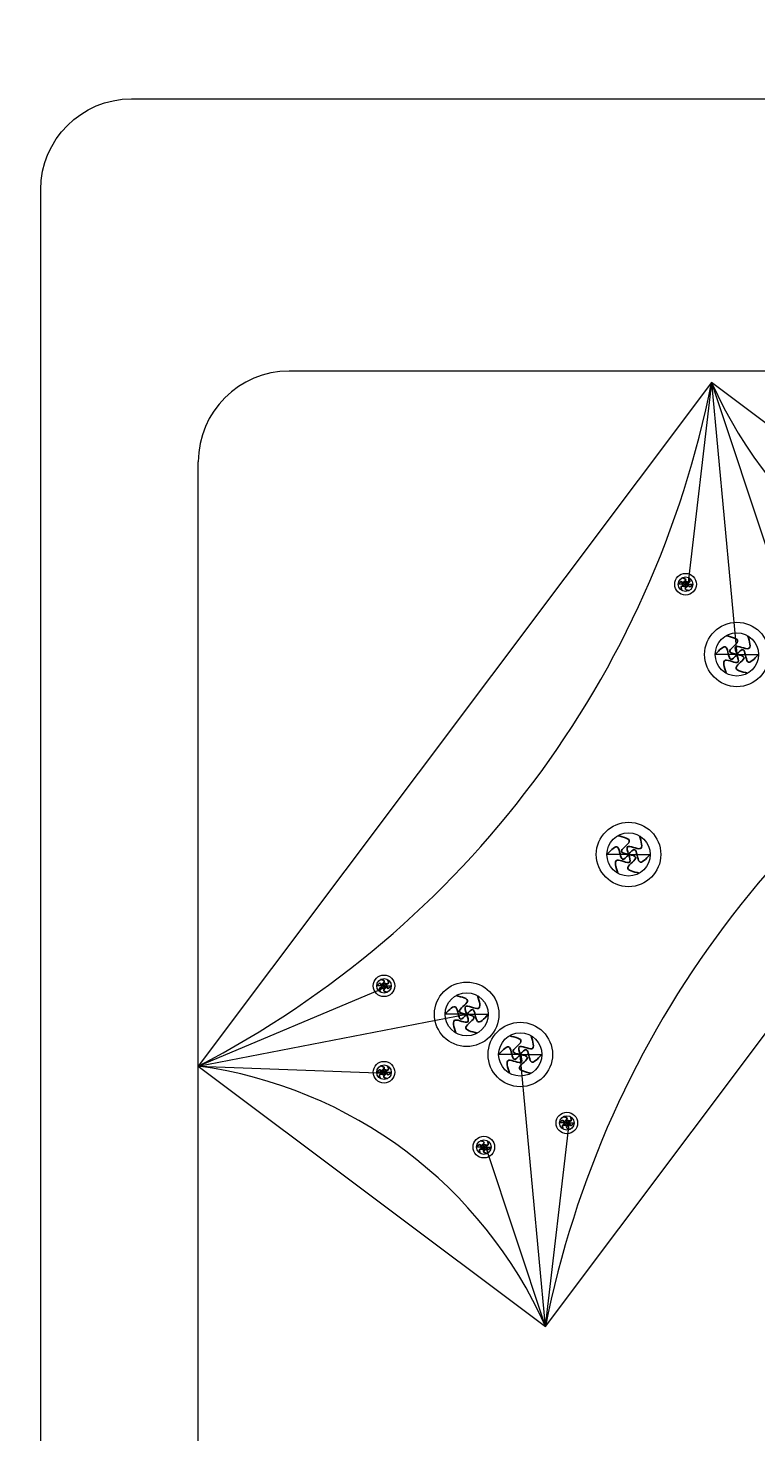
# Model space of a CAD drawing. Units: inches. Extents: x -61 to 1599, y -1316 to 257.
# Tile 103 of 204: x 126 to 142, y -99 to -68. Entities that reach past the tile are written whole.
import ezdxf

# ---------------------------------------------------------------- set-up
doc = ezdxf.new("R2010")
doc.units = ezdxf.units.IN
doc.header["$MEASUREMENT"] = 0
doc.layers.add('A-ANNO-DIMS', color=2, linetype='Continuous', lineweight=18)
doc.layers.add('FURNITURE', color=83, linetype='Continuous', lineweight=18)
doc.layers.add('FUR', color=83, linetype='Continuous')
doc.styles.get("Standard").update_dxf_attribs({"font": 'arial.ttf'})
doc.dimstyles.get("Standard").update_dxf_attribs({"dimtxt": 0.18, "dimasz": 0.18, "dimexe": 0.18, "dimexo": 0.0625, "dimgap": 0.09, "dimtad": 0, "dimtih": 1, "dimtoh": 1, "dimdec": 0, "dimzin": 0, "dimdsep": 46, "dimlunit": 3, "dimtxsty": 'Standard', "dimcen": 0.09, "dimadec": 0, "dimazin": 0, "dimtfac": 1, "dimtdec": 0, "dimtofl": 0, "dimtmove": 0, "dimatfit": 3, "dimfxl": 1, "dimtolj": 1, "dimtzin": 0, "dimarcsym": 0})

# ---------------------------------------------------------------- blocks, each defined once
blk = doc.blocks.new('*U186')
at = {"layer": 'FUR'}
blk.add_open_spline([(0.005, 0.08), (-0.03, 0.048), (-0.098, -0.015), (0.075, -0.018), (0.024, -0.063), (0.005, -0.08)], degree=3, knots=[0, 0, 0, 0, 0.0954578, 0.1898773, 0.2470677, 0.2470677, 0.2470677, 0.2470677], dxfattribs=at)
blk = doc.blocks.new('*U187')
at = {"layer": 'FUR', "transparency": 16777216}
for p, rotation in [((222.173, -79.977), 60), ((222.178, -80.056), 120), ((222.25, -80.092), 180), ((222.312, -79.968), 300), ((222.317, -80.048), 240)]:
    blk.add_blockref('*U186', p, dxfattribs=dict(at, rotation=rotation))
blk.add_blockref('*U186', (222.24, -79.932), dxfattribs=at)
blk = doc.blocks.new('*U198')
at = {"layer": 'FUR'}
blk.add_open_spline([(0.005, 0.08), (-0.03, 0.048), (-0.098, -0.015), (0.075, -0.018), (0.024, -0.063), (0.005, -0.08)], degree=3, knots=[0, 0, 0, 0, 0.0954578, 0.1898773, 0.2470677, 0.2470677, 0.2470677, 0.2470677], dxfattribs=at)
blk = doc.blocks.new('*U199')
at = {"layer": 'FUR', "transparency": 16777216}
for p, rotation in [((222.173, -79.977), 60), ((222.178, -80.056), 120), ((222.25, -80.092), 180), ((222.312, -79.968), 300), ((222.317, -80.048), 240)]:
    blk.add_blockref('*U198', p, dxfattribs=dict(at, rotation=rotation))
blk.add_blockref('*U198', (222.24, -79.932), dxfattribs=at)
blk = doc.blocks.new('*U210')
at = {"layer": 'FUR'}
blk.add_open_spline([(0.015, 0.238), (-0.088, 0.143), (-0.292, -0.045), (0.224, -0.053), (0.072, -0.187), (0.015, -0.238)], degree=3, knots=[0, 0, 0, 0, 0.2846533, 0.5662105, 0.736751, 0.736751, 0.736751, 0.736751], dxfattribs=at)
blk = doc.blocks.new('*U185')
at = {"layer": 'FUR', "transparency": 16777216}
blk.add_blockref('*U210', (662.716, -238.357), dxfattribs=at)
for p, rotation in [((662.929, -238.463), 300), ((662.517, -238.489), 60), ((662.531, -238.727), 120), ((662.944, -238.702), 240), ((662.745, -238.833), 180)]:
    blk.add_blockref('*U210', p, dxfattribs=dict(at, rotation=rotation))
blk = doc.blocks.new('*U200')
at = {"layer": 'FUR'}
blk.add_open_spline([(0.005, 0.08), (-0.03, 0.048), (-0.098, -0.015), (0.075, -0.018), (0.024, -0.063), (0.005, -0.08)], degree=3, knots=[0, 0, 0, 0, 0.0954578, 0.1898773, 0.2470677, 0.2470677, 0.2470677, 0.2470677], dxfattribs=at)
blk = doc.blocks.new('*U201')
at = {"layer": 'FUR', "transparency": 16777216}
for p, rotation in [((222.173, -79.977), 60), ((222.178, -80.056), 120), ((222.25, -80.092), 180), ((222.312, -79.968), 300), ((222.317, -80.048), 240)]:
    blk.add_blockref('*U200', p, dxfattribs=dict(at, rotation=rotation))
blk.add_blockref('*U200', (222.24, -79.932), dxfattribs=at)
blk = doc.blocks.new('*U194')
at = {"layer": 'FUR'}
blk.add_open_spline([(0.015, 0.238), (-0.088, 0.143), (-0.292, -0.045), (0.224, -0.053), (0.072, -0.187), (0.015, -0.238)], degree=3, knots=[0, 0, 0, 0, 0.2846533, 0.5662105, 0.736751, 0.736751, 0.736751, 0.736751], dxfattribs=at)
blk = doc.blocks.new('*U195')
at = {"layer": 'FUR', "transparency": 16777216}
blk.add_blockref('*U194', (662.716, -238.357), dxfattribs=at)
for p, rotation in [((662.929, -238.463), 300), ((662.517, -238.489), 60), ((662.531, -238.727), 120), ((662.944, -238.702), 240), ((662.745, -238.833), 180)]:
    blk.add_blockref('*U194', p, dxfattribs=dict(at, rotation=rotation))
blk = doc.blocks.new('*U202')
at = {"layer": 'FUR'}
blk.add_open_spline([(0.005, 0.08), (-0.03, 0.048), (-0.098, -0.015), (0.075, -0.018), (0.024, -0.063), (0.005, -0.08)], degree=3, knots=[0, 0, 0, 0, 0.0954578, 0.1898773, 0.2470677, 0.2470677, 0.2470677, 0.2470677], dxfattribs=at)
blk = doc.blocks.new('*U203')
at = {"layer": 'FUR', "transparency": 16777216}
for p, rotation in [((222.173, -79.977), 60), ((222.178, -80.056), 120), ((222.25, -80.092), 180), ((222.312, -79.968), 300), ((222.317, -80.048), 240)]:
    blk.add_blockref('*U202', p, dxfattribs=dict(at, rotation=rotation))
blk.add_blockref('*U202', (222.24, -79.932), dxfattribs=at)
blk = doc.blocks.new('*U196')
at = {"layer": 'FUR'}
blk.add_open_spline([(0.015, 0.238), (-0.088, 0.143), (-0.292, -0.045), (0.224, -0.053), (0.072, -0.187), (0.015, -0.238)], degree=3, knots=[0, 0, 0, 0, 0.2846533, 0.5662105, 0.736751, 0.736751, 0.736751, 0.736751], dxfattribs=at)
blk = doc.blocks.new('*U197')
at = {"layer": 'FUR', "transparency": 16777216}
blk.add_blockref('*U196', (662.716, -238.357), dxfattribs=at)
for p, rotation in [((662.929, -238.463), 300), ((662.517, -238.489), 60), ((662.531, -238.727), 120), ((662.944, -238.702), 240), ((662.745, -238.833), 180)]:
    blk.add_blockref('*U196', p, dxfattribs=dict(at, rotation=rotation))
blk = doc.blocks.new('*U190')
at = {"layer": 'FUR'}
blk.add_open_spline([(0.005, 0.08), (-0.03, 0.048), (-0.098, -0.015), (0.075, -0.018), (0.024, -0.063), (0.005, -0.08)], degree=3, knots=[0, 0, 0, 0, 0.0954578, 0.1898773, 0.2470677, 0.2470677, 0.2470677, 0.2470677], dxfattribs=at)
blk = doc.blocks.new('*U191')
at = {"layer": 'FUR', "transparency": 16777216}
for p, rotation in [((222.173, -79.977), 60), ((222.178, -80.056), 120), ((222.25, -80.092), 180), ((222.312, -79.968), 300), ((222.317, -80.048), 240)]:
    blk.add_blockref('*U190', p, dxfattribs=dict(at, rotation=rotation))
blk.add_blockref('*U190', (222.24, -79.932), dxfattribs=at)
blk = doc.blocks.new('*U209')
at = {"layer": 'FUR'}
blk.add_open_spline([(0.015, 0.238), (-0.088, 0.143), (-0.292, -0.045), (0.224, -0.053), (0.072, -0.187), (0.015, -0.238)], degree=3, knots=[0, 0, 0, 0, 0.2846533, 0.5662105, 0.736751, 0.736751, 0.736751, 0.736751], dxfattribs=at)
blk = doc.blocks.new('*U188')
at = {"layer": 'FUR', "transparency": 16777216}
blk.add_blockref('*U209', (662.716, -238.357), dxfattribs=at)
for p, rotation in [((662.929, -238.463), 300), ((662.517, -238.489), 60), ((662.531, -238.727), 120), ((662.944, -238.702), 240), ((662.745, -238.833), 180)]:
    blk.add_blockref('*U209', p, dxfattribs=dict(at, rotation=rotation))
blk = doc.blocks.new('SOFA-LOVESEAT')
for p, q in [((22.442, 54), (5.47, 54)), ((14.776, 53.751), (14.253, 49.285)), ((14.776, 53.751), (15.332, 47.757)), ((14.776, 53.751), (16.081, 49.817)), ((3.47, 8), (3.47, 52)), ((14.201, 49.305), (14.041, 49.305)), ((14.201, 49.305), (14.36, 49.305)), ((15.332, 47.757), (14.855, 47.757)), ((15.332, 47.757), (15.808, 47.757)), ((12.946, 43.35), (12.47, 43.35)), ((12.946, 43.35), (13.423, 43.35)), ((3.47, 38.686), (7.612, 40.436)), ((7.56, 40.455), (7.4, 40.455)), ((7.56, 40.455), (7.719, 40.455)), ((3.47, 38.686), (9.381, 39.828)), ((9.381, 39.828), (8.904, 39.828)), ((9.381, 39.828), (9.857, 39.828)), ((3.47, 38.686), (7.612, 38.532)), ((10.561, 38.942), (10.084, 38.942)), ((11.116, 32.948), (10.561, 38.942)), ((10.561, 38.942), (11.037, 38.942)), ((7.56, 38.551), (7.4, 38.551)), ((7.56, 38.551), (7.719, 38.551)), ((11.587, 37.433), (11.427, 37.433)), ((11.587, 37.433), (11.747, 37.433)), ((11.116, 32.948), (11.639, 37.414)), ((9.759, 36.901), (9.599, 36.901)), ((9.759, 36.901), (9.918, 36.901)), ((11.116, 32.948), (9.811, 36.882))]:
    blk.add_line(p, q)
blk.add_lwpolyline([(26, 6), (26, 2, -0.414214), (24, 0), (2, 0, -0.414214), (0, 2), (0, 58, -0.414213), (2, 60), (24, 60, -0.414214), (26, 58), (26, 54)], format="xyb")
blk.add_lwpolyline([(11.116, 32.948), (22.422, 48.013), (14.776, 53.751), (3.47, 38.686)], close=True)
for centre, radius in [((14.201, 49.305), 0.238), ((14.201, 49.305), 0.16), ((15.332, 47.757), 0.71), ((15.332, 47.757), 0.476), ((12.946, 43.35), 0.71), ((12.946, 43.35), 0.476), ((7.56, 40.455), 0.238), ((7.56, 40.455), 0.16), ((9.381, 39.828), 0.71), ((9.381, 39.828), 0.476), ((10.561, 38.942), 0.71), ((10.561, 38.942), 0.476), ((7.56, 38.551), 0.238), ((7.56, 38.551), 0.16), ((11.587, 37.433), 0.238), ((11.587, 37.433), 0.16), ((9.759, 36.901), 0.238), ((9.759, 36.901), 0.16)]:
    blk.add_circle(centre, radius)
for centre, radius, start, end in [((5.47, 52), 2, 90, 180), ((-6.541, 57.974), 21.731, 297.4317, 348.7956), ((23.745, 57.74), 9.816, 203.9742, 262.253), ((32.433, 28.726), 21.731, 117.4317, 168.7956), ((2.147, 28.96), 9.816, 23.9742, 82.253)]:
    blk.add_arc(centre, radius, start, end)
at = {"xscale": -1, "rotation": 90.00003000000098}
for name, p in [('*U191', (-65.812, 271.55)), ('*U188', (-223.264, 710.487)), ('*U197', (-225.649, 706.08)), ('*U187', (-72.453, 262.7)), ('*U185', (-229.215, 702.558)), ('*U195', (-228.035, 701.672)), ('*U199', (-72.453, 260.796)), ('*U203', (-68.426, 259.678)), ('*U201', (-70.254, 259.146))]:
    blk.add_blockref(name, p, dxfattribs=at)
blk = doc.blocks.new('*D687')
at = {"layer": 'A-ANNO-DIMS', "color": 0, "lineweight": -2, "transparency": 16777216}
for p, q in [((289.418, 181.677), (-61.077, 181.677)), ((-60.897, 181.497), (-60.897, -528.952)), ((-60.897, -1239.765), (-60.897, -529.316)), ((319.64, -1239.945), (-61.077, -1239.945))]:
    blk.add_line(p, q, dxfattribs=at)
at = {"layer": 'A-ANNO-DIMS', "color": 0, "transparency": 16777216}
for points in [[(-60.927, 181.497), (-60.867, 181.497), (-60.897, 181.677)], [(-60.927, -1239.765), (-60.867, -1239.765), (-60.897, -1239.945)]]:
    blk.add_solid(points, dxfattribs=at)
at = {"layer": 'DEFPOINTS', "color": 0, "transparency": 16777216}
for p in [(289.481, 181.677), (-60.897, -1239.945), (319.703, -1239.945)]:
    blk.add_point(p, dxfattribs=at)
at = {"layer": 'A-ANNO-DIMS', "color": 0, "transparency": 16777216, "insert": (-60.897, -529.134), "char_height": 0.18, "attachment_point": 5}
blk.add_mtext('\\A1;1421.6', dxfattribs=at)
blk = doc.blocks.new('*D700')
at = {"layer": 'A-ANNO-DIMS', "color": 0, "lineweight": -2, "transparency": 16777216}
for p, q in [((14.703, -616.882), (14.703, 257.457)), ((179.752, -616.882), (179.752, 257.457)), ((14.883, 257.277), (96.772, 257.277)), ((179.572, 257.277), (97.683, 257.277))]:
    blk.add_line(p, q, dxfattribs=at)
at = {"layer": 'A-ANNO-DIMS', "color": 0, "transparency": 16777216}
for points in [[(14.883, 257.307), (14.883, 257.247), (14.703, 257.277)], [(179.572, 257.307), (179.572, 257.247), (179.752, 257.277)]]:
    blk.add_solid(points, dxfattribs=at)
at = {"layer": 'DEFPOINTS', "color": 0, "transparency": 16777216}
for p in [(179.752, 257.277), (14.703, -616.945), (179.752, -616.945)]:
    blk.add_point(p, dxfattribs=at)
at = {"layer": 'A-ANNO-DIMS', "color": 0, "transparency": 16777216, "insert": (97.227, 257.277), "char_height": 0.18, "attachment_point": 5}
blk.add_mtext('\\A1;165.05', dxfattribs=at)

msp = doc.modelspace()

# ---------------------------------------------------------------- block references
at = {"layer": 'FURNITURE'}
msp.add_blockref('SOFA-LOVESEAT', (125.901, -129.695), dxfattribs=at)

# ---------------------------------------------------------------- dimensions: what is measured, and where the dimension line sits
at = {"layer": 'A-ANNO-DIMS'}
dim = msp.add_linear_dim(base=(179.7521, 257.2771), p1=(14.7028, -616.9446), p2=(179.7521, -616.9446), dimstyle='Standard', override={"dimdec": 2, "dimlfac": 1, "dimrnd": 0, "dimzin": 0, "dimdsep": 46, "dimlunit": 2}, dxfattribs=at)
dim.commit()
dim.dimension.update_dxf_attribs({"geometry": '*D700', "text_midpoint": (97.2274, 257.2771)})
dim = msp.add_linear_dim(base=(-60.8972, -1239.9446), p1=(289.4807, 181.6771), p2=(319.7028, -1239.9446), angle=90, dimstyle='Standard', override={"dimdec": 1, "dimlfac": 1, "dimrnd": 0, "dimzin": 0, "dimdsep": 46, "dimlunit": 2}, dxfattribs=at)
dim.commit()
dim.dimension.update_dxf_attribs({"geometry": '*D687', "text_midpoint": (-60.8972, -529.1337)})

doc.saveas('drawing.dxf')
